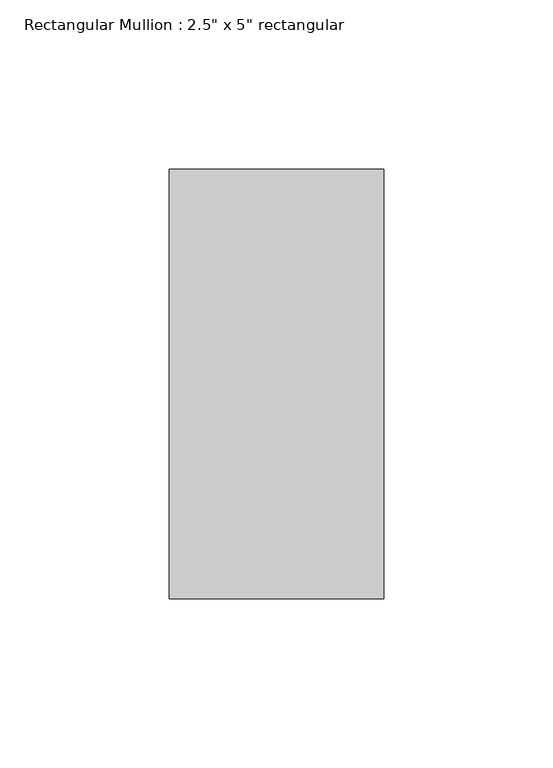
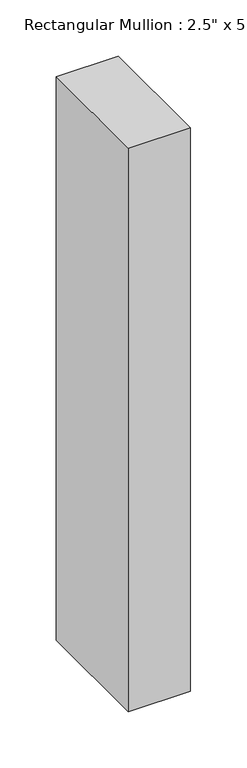
"""IFC4 building model written with IfcOpenShell, lengths in millimetres: member geometry."""

from ifc_helpers import new_model, si_unit, frame, origin, place, context, project, spatial, polyline, outline, extrude, source, transform, mapped, element, save


def member_6e77e263(model_context):
    return source(origin(), model_context, "Body", "SweptSolid", [
        extrude(outline(polyline([(31.75, 63.5), (31.75, -63.5), (-31.75, -63.5), (-31.75, 63.5), (31.75, 63.5)])), frame((0.0, 0.0, -609.6), z_axis=(0.0, 0.0, 1.0), x_axis=(1.0, 0.0, 0.0)), (0.0, 0.0, 1.0), 609.6),
    ])


if __name__ == "__main__":
    model = new_model("IFC4")
    model_context = context("Model", 3, world=origin())
    ifc_project = project(units=[si_unit("LENGTHUNIT", "METRE", prefix="MILLI")], contexts=[model_context])
    site = spatial("IfcSite", under=ifc_project)
    building = spatial("IfcBuilding", under=site)
    placement = place(None, origin())
    member_shape = member_6e77e263(model_context)
    element("IfcMember", 1, ObjectType="Rectangular Mullion : 2.5\" x 5\" rectangular", at=placement, inside=building, context=model_context, shape_type="MappedRepresentation", body=[
        mapped(member_shape, transform((0.0, 0.0, 0.0), x_axis=(1.0, 0.0, 0.0), y_axis=(0.0, 1.0, 0.0), z_axis=(0.0, 0.0, 1.0))),
    ])
    save(model, "model.ifc")

# Revit data of these elements
# Type "Rectangular Mullion : 2.5\" x 5\" rectangular"
#   built-in parameter 1007304 = 0.416667 (stored number, unit not read)
#   built-in parameter 1007301 = 0.104167 (stored number, unit not read)
#   built-in parameter 1007300 = 0.104167 (stored number, unit not read)
